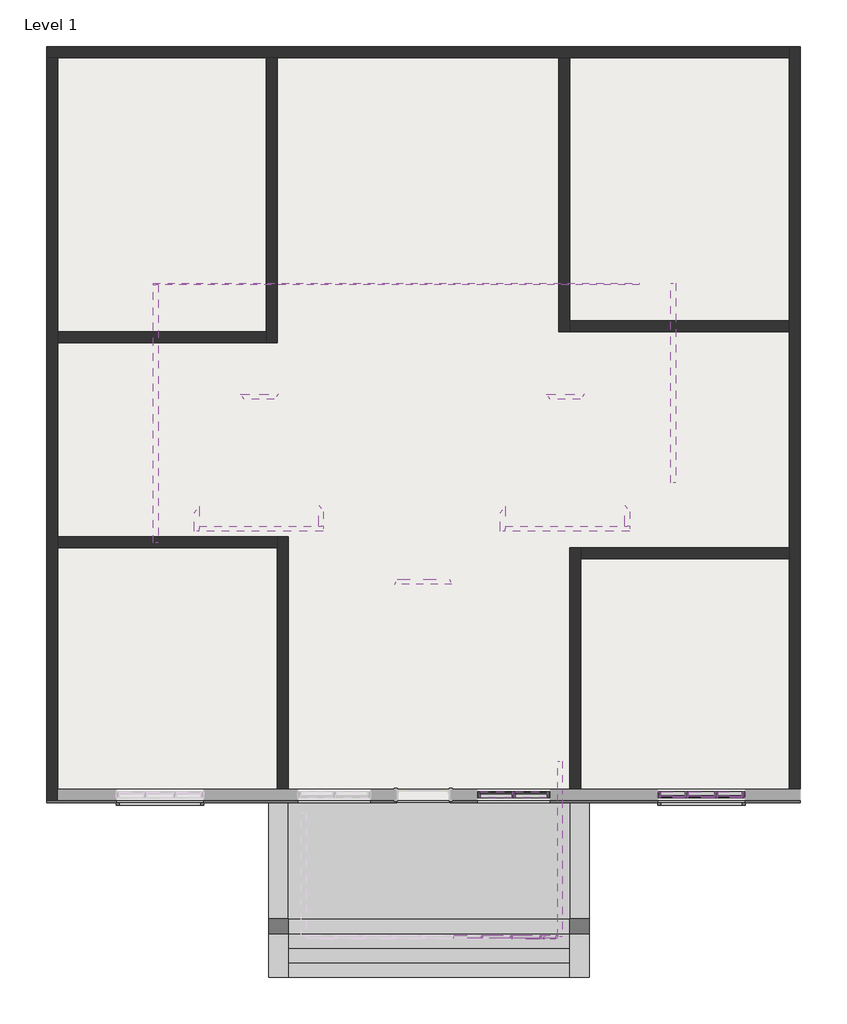
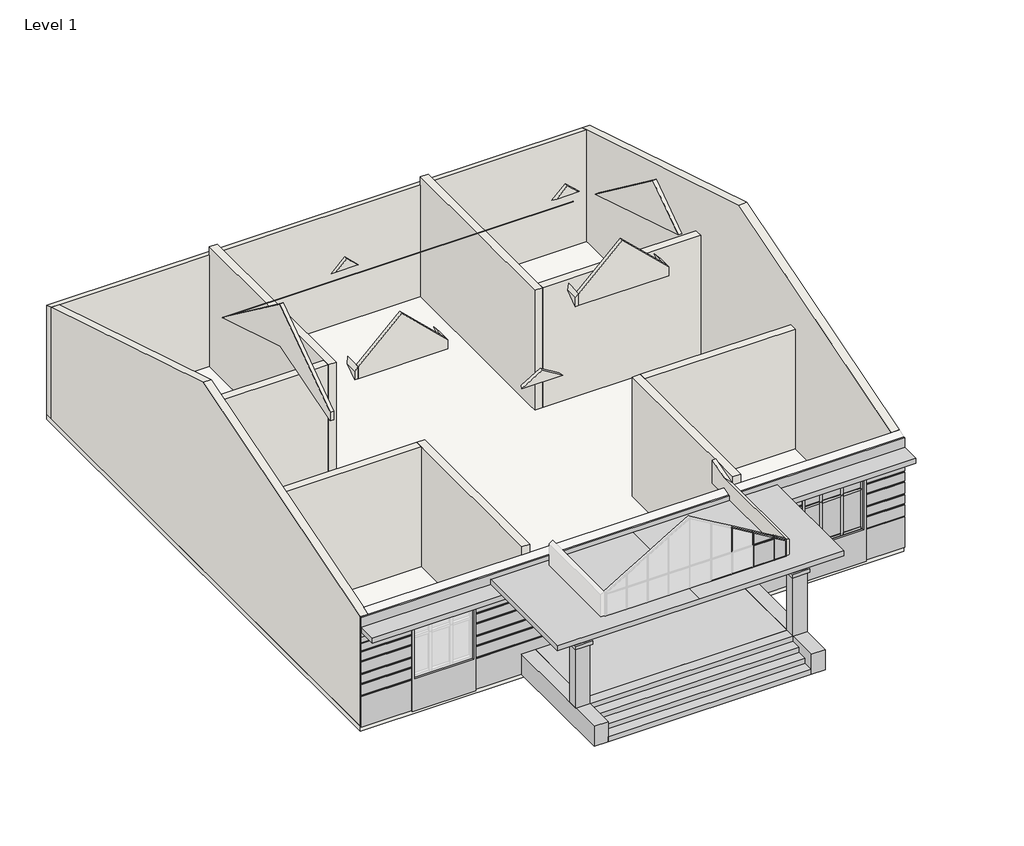
# One storey, part 2 of 2: 38 members, 24 walls, 11 plates, 1 proxy, 1 slab.
"""IFC4 building model written with IfcOpenShell, lengths in millimetres."""

from ifc_helpers import new_model, si_unit, frame, origin, origin_with_axes, place, context, project, spatial, polyline, outline, extrude, faceted_brep, transform, mapped, element, save
from components import generic_models_1_generic_models_1_130779d0, member_b22cb31b, member_1ff0c156, member_6458fcce, member_a67f877f, member_f89b2291, member_594eddbe, member_fdc2508a, member_99ded25b, member_354dc74f, member_6356c2c7, member_864d0aaa, member_0b7646a3, member_2b49869a, member_aaa03826, member_0a1a1ade, member_a980948f, member_6e77e263, member_47bfaf8a, member_75074519, member_c33c434a, member_38e9bff8, member_062c1ce8, system_panel_glazed_d796fc41, system_panel_glazed_2d0a2ff2, system_panel_glazed_c086748d, system_panel_glazed_4278ab3a, system_panel_glazed_31f7001e, system_panel_glazed_2554e476, system_panel_glazed_f02c31ce, system_panel_glazed_28184e5f

model = new_model("IFC4")

# Units and contexts
model_context = context("Model", 3, world=origin())
ifc_project = project(units=[si_unit("LENGTHUNIT", "METRE", prefix="MILLI")], contexts=[model_context])

# Site, building, storey
site = spatial("IfcSite", under=ifc_project)
building = spatial("IfcBuilding", under=site)
storey = spatial("IfcBuildingStorey", under=building, Name="Level 1", Elevation=0.0)

# Proxy
placement = place(None, origin())
generic_models_1_generic_models_1_shape = generic_models_1_generic_models_1_130779d0(model_context)
element("IfcBuildingElementProxy", 1, Name="Generic Models 1 : Generic Models 1", ObjectType="Generic Models 1 : Generic Models 1", at=placement, inside=storey, context=model_context, shape_type="MappedRepresentation", body=[
    mapped(generic_models_1_generic_models_1_shape, transform((0.0, 0.0, 0.0), x_axis=(1.0, 0.0, 0.0), y_axis=(0.0, 1.0, 0.0), z_axis=(0.0, 0.0, 1.0))),
])

# Members
member_shape = member_b22cb31b(model_context)
element("IfcMember", 2, ObjectType="Rectangular Mullion : 1.5\" x 2.5\" rectangular", at=placement, inside=storey, context=model_context, shape_type="MappedRepresentation", body=[
    mapped(member_shape, transform((1849.2182444, -4522.7940778, 3200.4), x_axis=(0.0, 0.0, -1.0), y_axis=(0.0, 1.0, 0.0), z_axis=(1.0, 0.0, 0.0))),
])
member_2_shape = member_1ff0c156(model_context)
element("IfcMember", 3, ObjectType="Rectangular Mullion : 1.5\" x 2.5\" rectangular", at=placement, inside=storey, context=model_context, shape_type="MappedRepresentation", body=[
    mapped(member_2_shape, transform((1551.6847658, -4522.7940778, 3886.2), x_axis=(0.0, 0.0, 1.0), y_axis=(0.0, 1.0, 0.0), z_axis=(-1.0, 0.0, 0.0))),
])
member_3_shape = member_6458fcce(model_context)
element("IfcMember", 4, ObjectType="Rectangular Mullion : 1.5\" x 2.5\" rectangular", at=placement, inside=storey, context=model_context, shape_type="MappedRepresentation", body=[
    mapped(member_3_shape, transform((1532.6347658, -4522.7940778, 3200.4), x_axis=(-1.0, 0.0, 0.0), y_axis=(0.0, 1.0, 0.0), z_axis=(0.0, 0.0, -1.0))),
])
member_4_shape = member_a67f877f(model_context)
element("IfcMember", 5, ObjectType="Rectangular Mullion : 1.5\" x 2.5\" rectangular", at=placement, inside=storey, context=model_context, shape_type="MappedRepresentation", body=[
    mapped(member_4_shape, transform((294.3847658, -4522.7940778, 3200.4), x_axis=(0.0, 0.0, -1.0), y_axis=(0.0, 1.0, 0.0), z_axis=(1.0, 0.0, 0.0))),
])
element("IfcMember", 6, ObjectType="Rectangular Mullion : 1.5\" x 2.5\" rectangular", at=placement, inside=storey, context=model_context, shape_type="MappedRepresentation", body=[
    mapped(member_4_shape, transform((903.9847658, -4522.7940778, 3200.4), x_axis=(0.0, 0.0, -1.0), y_axis=(0.0, 1.0, 0.0), z_axis=(1.0, 0.0, 0.0))),
])
element("IfcMember", 7, ObjectType="Rectangular Mullion : 1.5\" x 2.5\" rectangular", at=placement, inside=storey, context=model_context, shape_type="MappedRepresentation", body=[
    mapped(member_4_shape, transform((1513.5847658, -4522.7940778, 3200.4), x_axis=(0.0, 0.0, -1.0), y_axis=(0.0, 1.0, 0.0), z_axis=(1.0, 0.0, 0.0))),
])
member_5_shape = member_f89b2291(model_context)
element("IfcMember", 8, ObjectType="Rectangular Mullion : 1.5\" x 2.5\" rectangular", at=placement, inside=storey, context=model_context, shape_type="MappedRepresentation", body=[
    mapped(member_5_shape, transform((1617.4006914, -4522.7940778, 3886.2), x_axis=(0.5109163571310299, 0.0, 0.8596304299034312), y_axis=(0.0, 1.0, 0.0), z_axis=(-0.8596304299034312, 0.0, 0.5109163571310299))),
])
member_6_shape = member_594eddbe(model_context)
element("IfcMember", 9, ObjectType="Rectangular Mullion : 1.5\" x 2.5\" rectangular", at=placement, inside=storey, context=model_context, shape_type="MappedRepresentation", body=[
    mapped(member_6_shape, transform((313.4347658, -4522.7940778, 4661.2045803), x_axis=(0.5109163571310306, 0.0, 0.8596304299034309), y_axis=(0.0, 1.0, 0.0), z_axis=(-0.8596304299034307, 0.0, 0.5109163571310305))),
])
element("IfcMember", 10, ObjectType="Rectangular Mullion : 1.5\" x 2.5\" rectangular", at=placement, inside=storey, context=model_context, shape_type="MappedRepresentation", body=[
    mapped(member_6_shape, transform((923.0347658, -4522.7940778, 4298.8923581), x_axis=(0.5109163571310307, 0.0, 0.8596304299034307), y_axis=(0.0, 1.0, 0.0), z_axis=(-0.8596304299034307, 0.0, 0.5109163571310307))),
])
member_7_shape = member_fdc2508a(model_context)
element("IfcMember", 11, ObjectType="Rectangular Mullion : 1.5\" x 2.5\" rectangular", at=placement, inside=storey, context=model_context, shape_type="MappedRepresentation", body=[
    mapped(member_7_shape, transform((1532.6347658, -4522.7940778, 3936.5801359), x_axis=(0.5109163571310298, 0.0, 0.8596304299034313), y_axis=(0.0, 1.0, 0.0), z_axis=(-0.8596304299034312, 0.0, 0.5109163571310297))),
])
member_8_shape = member_99ded25b(model_context)
element("IfcMember", 12, ObjectType="Rectangular Mullion : 1.5\" x 2.5\" rectangular", at=placement, inside=storey, context=model_context, shape_type="MappedRepresentation", body=[
    mapped(member_8_shape, transform((313.4347658, -4522.7940778, 3886.2), x_axis=(-1.0, 0.0, 0.0), y_axis=(0.0, 1.0, 0.0), z_axis=(0.0, 0.0, -1.0))),
])
member_9_shape = member_354dc74f(model_context)
element("IfcMember", 13, ObjectType="Rectangular Mullion : 1.5\" x 2.5\" rectangular", at=placement, inside=storey, context=model_context, shape_type="MappedRepresentation", body=[
    mapped(member_9_shape, transform((923.0347658, -4522.7940778, 3886.2), x_axis=(-1.0, 0.0, 0.0), y_axis=(0.0, 1.0, 0.0), z_axis=(0.0, 0.0, -1.0))),
])
member_10_shape = member_6356c2c7(model_context)
element("IfcMember", 14, ObjectType="Rectangular Mullion : 1.5\" x 2.5\" rectangular", at=placement, inside=storey, context=model_context, shape_type="MappedRepresentation", body=[
    mapped(member_10_shape, transform((1532.6347658, -4522.7940778, 3886.2), x_axis=(-1.0, 0.0, 0.0), y_axis=(0.0, 1.0, 0.0), z_axis=(0.0, 0.0, -1.0))),
])
member_11_shape = member_864d0aaa(model_context)
element("IfcMember", 15, ObjectType="Rectangular Mullion : 1.5\" x 2.5\" rectangular", at=placement, inside=storey, context=model_context, shape_type="MappedRepresentation", body=[
    mapped(member_11_shape, transform((1887.3182444, -4522.7940778, 3725.7760689), x_axis=(1.0, 0.0, 0.0), y_axis=(0.0, 1.0, 0.0), z_axis=(0.0, 0.0, 1.0))),
])
member_12_shape = member_0b7646a3(model_context)
element("IfcMember", 16, ObjectType="Rectangular Mullion : 2.5\" x 5\" rectangular", at=placement, inside=storey, context=model_context, shape_type="MappedRepresentation", body=[
    mapped(member_12_shape, transform((4034.5347658, -1562.8594336, 2743.2), x_axis=(0.0, 0.0, 1.0), y_axis=(0.0, 1.0, 0.0), z_axis=(-1.0, 0.0, 0.0))),
])
element("IfcMember", 17, ObjectType="Rectangular Mullion : 2.5\" x 5\" rectangular", at=placement, inside=storey, context=model_context, shape_type="MappedRepresentation", body=[
    mapped(member_12_shape, transform((5221.9847658, -1562.8594336, 2743.2), x_axis=(0.0, 0.0, 1.0), y_axis=(0.0, 1.0, 0.0), z_axis=(-1.0, 0.0, 0.0))),
])
element("IfcMember", 18, ObjectType="Rectangular Mullion : 2.5\" x 5\" rectangular", at=placement, inside=storey, context=model_context, shape_type="MappedRepresentation", body=[
    mapped(member_12_shape, transform((5736.3347658, -1562.8594336, 914.4), x_axis=(0.0, 0.0, -1.0), y_axis=(0.0, 1.0, 0.0), z_axis=(1.0, 0.0, 0.0))),
])
element("IfcMember", 19, ObjectType="Rectangular Mullion : 2.5\" x 5\" rectangular", at=placement, inside=storey, context=model_context, shape_type="MappedRepresentation", body=[
    mapped(member_12_shape, transform((4548.8847658, -1562.8594336, 914.4), x_axis=(0.0, 0.0, -1.0), y_axis=(0.0, 1.0, 0.0), z_axis=(1.0, 0.0, 0.0))),
])
member_13_shape = member_2b49869a(model_context)
element("IfcMember", 20, ObjectType="Rectangular Mullion : 2.5\" x 5\" rectangular", at=placement, inside=storey, context=model_context, shape_type="MappedRepresentation", body=[
    mapped(member_13_shape, transform((4580.6347658, -1562.8594336, 914.4), x_axis=(-1.0, 0.0, 0.0), y_axis=(0.0, 1.0, 0.0), z_axis=(0.0, 0.0, -1.0))),
])
element("IfcMember", 21, ObjectType="Rectangular Mullion : 2.5\" x 5\" rectangular", at=placement, inside=storey, context=model_context, shape_type="MappedRepresentation", body=[
    mapped(member_13_shape, transform((5190.2347658, -1562.8594336, 914.4), x_axis=(-1.0, 0.0, 0.0), y_axis=(0.0, 1.0, 0.0), z_axis=(0.0, 0.0, -1.0))),
])
member_14_shape = member_aaa03826(model_context)
element("IfcMember", 22, ObjectType="Rectangular Mullion : 2.5\" x 5\" rectangular", at=placement, inside=storey, context=model_context, shape_type="MappedRepresentation", body=[
    mapped(member_14_shape, transform((5221.9847658, -1562.8594336, 2133.6), x_axis=(0.0, 0.0, 1.0), y_axis=(0.0, 1.0, 0.0), z_axis=(-1.0, 0.0, 0.0))),
])
element("IfcMember", 23, ObjectType="Rectangular Mullion : 2.5\" x 5\" rectangular", at=placement, inside=storey, context=model_context, shape_type="MappedRepresentation", body=[
    mapped(member_14_shape, transform((4034.5347658, -1562.8594336, 2133.6), x_axis=(0.0, 0.0, 1.0), y_axis=(0.0, 1.0, 0.0), z_axis=(-1.0, 0.0, 0.0))),
])
member_15_shape = member_0a1a1ade(model_context)
element("IfcMember", 24, ObjectType="Rectangular Mullion : 2.5\" x 5\" rectangular", at=placement, inside=storey, context=model_context, shape_type="MappedRepresentation", body=[
    mapped(member_15_shape, transform((4612.3847658, -1562.8594336, 2133.6), x_axis=(0.0, 0.0, 1.0), y_axis=(0.0, 1.0, 0.0), z_axis=(-1.0, 0.0, 0.0))),
])
member_16_shape = member_a980948f(model_context)
element("IfcMember", 25, ObjectType="Rectangular Mullion : 2.5\" x 5\" rectangular", at=placement, inside=storey, context=model_context, shape_type="MappedRepresentation", body=[
    mapped(member_16_shape, transform((5158.4847658, -1562.8594336, 914.4), x_axis=(0.0, 0.0, -1.0), y_axis=(0.0, 1.0, 0.0), z_axis=(1.0, 0.0, 0.0))),
])
element("IfcMember", 26, ObjectType="Rectangular Mullion : 2.5\" x 5\" rectangular", at=placement, inside=storey, context=model_context, shape_type="MappedRepresentation", body=[
    mapped(member_16_shape, transform((4612.3847658, -1562.8594336, 2743.2), x_axis=(0.0, 0.0, 1.0), y_axis=(0.0, 1.0, 0.0), z_axis=(-1.0, 0.0, 0.0))),
])
member_17_shape = member_6e77e263(model_context)
element("IfcMember", 27, ObjectType="Rectangular Mullion : 2.5\" x 5\" rectangular", at=placement, inside=storey, context=model_context, shape_type="MappedRepresentation", body=[
    mapped(member_17_shape, transform((4580.6347658, -1562.8594336, 2133.6), x_axis=(-1.0, 0.0, 0.0), y_axis=(0.0, 1.0, 0.0), z_axis=(0.0, 0.0, -1.0))),
])
element("IfcMember", 28, ObjectType="Rectangular Mullion : 2.5\" x 5\" rectangular", at=placement, inside=storey, context=model_context, shape_type="MappedRepresentation", body=[
    mapped(member_17_shape, transform((5190.2347658, -1562.8594336, 2133.6), x_axis=(-1.0, 0.0, 0.0), y_axis=(0.0, 1.0, 0.0), z_axis=(0.0, 0.0, -1.0))),
])
member_18_shape = member_47bfaf8a(model_context)
element("IfcMember", 29, ObjectType="Rectangular Mullion : 2.5\" x 5\" rectangular", at=placement, inside=storey, context=model_context, shape_type="MappedRepresentation", body=[
    mapped(member_18_shape, transform((5799.8347658, -1562.8594336, 2743.2), x_axis=(1.0, 0.0, 0.0), y_axis=(0.0, 1.0, 0.0), z_axis=(0.0, 0.0, 1.0))),
])
member_19_shape = member_75074519(model_context)
element("IfcMember", 30, ObjectType="Rectangular Mullion : 2.5\" x 5\" rectangular", at=placement, inside=storey, context=model_context, shape_type="MappedRepresentation", body=[
    mapped(member_19_shape, transform((3971.0347658, -1562.8594336, 914.4), x_axis=(-1.0, 0.0, 0.0), y_axis=(0.0, 1.0, 0.0), z_axis=(0.0, 0.0, -1.0))),
])
element("IfcMember", 31, ObjectType="Rectangular Mullion : 2.5\" x 5\" rectangular", at=placement, inside=storey, context=model_context, shape_type="MappedRepresentation", body=[
    mapped(member_18_shape, transform((3971.0347658, -1562.8594336, 2133.6), x_axis=(-1.0, 0.0, 0.0), y_axis=(0.0, 1.0, 0.0), z_axis=(0.0, 0.0, -1.0))),
])
element("IfcMember", 32, ObjectType="Rectangular Mullion : 2.5\" x 5\" rectangular", at=placement, inside=storey, context=model_context, shape_type="MappedRepresentation", body=[
    mapped(member_19_shape, transform((5799.8347658, -1562.8594336, 2133.6), x_axis=(1.0, 0.0, 0.0), y_axis=(0.0, 1.0, 0.0), z_axis=(0.0, 0.0, 1.0))),
])
member_20_shape = member_c33c434a(model_context)
element("IfcMember", 33, ObjectType="Rectangular Mullion : 2.5\" x 5\" rectangular", at=placement, inside=storey, context=model_context, shape_type="MappedRepresentation", body=[
    mapped(member_20_shape, transform((1672.3347658, -1562.8594336, 2743.2), x_axis=(0.0, 0.0, 1.0), y_axis=(0.0, -1.0, 0.0), z_axis=(1.0, 0.0, 0.0))),
])
element("IfcMember", 34, ObjectType="Rectangular Mullion : 2.5\" x 5\" rectangular", at=placement, inside=storey, context=model_context, shape_type="MappedRepresentation", body=[
    mapped(member_20_shape, transform((942.0847658, -1562.8594336, 2743.2), x_axis=(0.0, 0.0, 1.0), y_axis=(0.0, -1.0, 0.0), z_axis=(1.0, 0.0, 0.0))),
])
element("IfcMember", 35, ObjectType="Rectangular Mullion : 2.5\" x 5\" rectangular", at=placement, inside=storey, context=model_context, shape_type="MappedRepresentation", body=[
    mapped(member_20_shape, transform((275.3347658, -1562.8594336, 1066.8), x_axis=(0.0, 0.0, -1.0), y_axis=(0.0, -1.0, 0.0), z_axis=(-1.0, 0.0, 0.0))),
])
element("IfcMember", 36, ObjectType="Rectangular Mullion : 2.5\" x 5\" rectangular", at=placement, inside=storey, context=model_context, shape_type="MappedRepresentation", body=[
    mapped(member_20_shape, transform((1005.5847658, -1562.8594336, 1066.8), x_axis=(0.0, 0.0, -1.0), y_axis=(0.0, -1.0, 0.0), z_axis=(-1.0, 0.0, 0.0))),
])
member_21_shape = member_38e9bff8(model_context)
element("IfcMember", 37, ObjectType="Rectangular Mullion : 2.5\" x 5\" rectangular", at=placement, inside=storey, context=model_context, shape_type="MappedRepresentation", body=[
    mapped(member_21_shape, transform((973.8347658, -1562.8594336, 1066.8), x_axis=(1.0, 0.0, 0.0), y_axis=(0.0, -1.0, 0.0), z_axis=(0.0, 0.0, -1.0))),
])
member_22_shape = member_062c1ce8(model_context)
element("IfcMember", 38, ObjectType="Rectangular Mullion : 2.5\" x 5\" rectangular", at=placement, inside=storey, context=model_context, shape_type="MappedRepresentation", body=[
    mapped(member_22_shape, transform((211.8347658, -1562.8594336, 2743.2), x_axis=(-1.0, 0.0, 0.0), y_axis=(0.0, -1.0, 0.0), z_axis=(0.0, 0.0, 1.0))),
])
element("IfcMember", 39, ObjectType="Rectangular Mullion : 2.5\" x 5\" rectangular", at=placement, inside=storey, context=model_context, shape_type="MappedRepresentation", body=[
    mapped(member_22_shape, transform((1735.8347658, -1562.8594336, 1066.8), x_axis=(1.0, 0.0, 0.0), y_axis=(0.0, -1.0, 0.0), z_axis=(0.0, 0.0, -1.0))),
])

# Plates
system_panel_glazed_shape = system_panel_glazed_d796fc41(model_context)
element("IfcPlate", 40, ObjectType="System Panel : Glazed", at=placement, inside=storey, context=model_context, shape_type="MappedRepresentation", body=[
    mapped(system_panel_glazed_shape, transform((5479.1597658, -1562.8594336, 977.9), x_axis=(-1.0, 0.0, 0.0), y_axis=(0.0, -1.0, 0.0), z_axis=(0.0, 0.0, 1.0))),
])
element("IfcPlate", 41, ObjectType="System Panel : Glazed", at=placement, inside=storey, context=model_context, shape_type="MappedRepresentation", body=[
    mapped(system_panel_glazed_shape, transform((4291.7097658, -1562.8594336, 977.9), x_axis=(-1.0, 0.0, 0.0), y_axis=(0.0, -1.0, 0.0), z_axis=(0.0, 0.0, 1.0))),
])
system_panel_glazed_2_shape = system_panel_glazed_2d0a2ff2(model_context)
element("IfcPlate", 42, ObjectType="System Panel : Glazed", at=placement, inside=storey, context=model_context, shape_type="MappedRepresentation", body=[
    mapped(system_panel_glazed_2_shape, transform((4885.4347658, -1562.8594336, 977.9), x_axis=(-1.0, 0.0, 0.0), y_axis=(0.0, -1.0, 0.0), z_axis=(0.0, 0.0, 1.0))),
])
system_panel_glazed_3_shape = system_panel_glazed_c086748d(model_context)
element("IfcPlate", 43, ObjectType="System Panel : Glazed", at=placement, inside=storey, context=model_context, shape_type="MappedRepresentation", body=[
    mapped(system_panel_glazed_3_shape, transform((5479.1597658, -1562.8594336, 2165.35), x_axis=(-1.0, 0.0, 0.0), y_axis=(0.0, -1.0, 0.0), z_axis=(0.0, 0.0, 1.0))),
])
element("IfcPlate", 44, ObjectType="System Panel : Glazed", at=placement, inside=storey, context=model_context, shape_type="MappedRepresentation", body=[
    mapped(system_panel_glazed_3_shape, transform((4291.7097658, -1562.8594336, 2165.35), x_axis=(-1.0, 0.0, 0.0), y_axis=(0.0, -1.0, 0.0), z_axis=(0.0, 0.0, 1.0))),
])
system_panel_glazed_4_shape = system_panel_glazed_4278ab3a(model_context)
element("IfcPlate", 45, ObjectType="System Panel : Glazed", at=placement, inside=storey, context=model_context, shape_type="MappedRepresentation", body=[
    mapped(system_panel_glazed_4_shape, transform((4885.4347658, -1562.8594336, 2165.35), x_axis=(-1.0, 0.0, 0.0), y_axis=(0.0, -1.0, 0.0), z_axis=(0.0, 0.0, 1.0))),
])
system_panel_glazed_5_shape = system_panel_glazed_31f7001e(model_context)
element("IfcPlate", 46, ObjectType="System Panel : Glazed", at=placement, inside=storey, context=model_context, shape_type="MappedRepresentation", body=[
    mapped(system_panel_glazed_5_shape, transform((608.7097658, -1562.8594336, 1130.3), x_axis=(1.0, 0.0, 0.0), y_axis=(0.0, 1.0, 0.0), z_axis=(0.0, 0.0, 1.0))),
])
element("IfcPlate", 47, ObjectType="System Panel : Glazed", at=placement, inside=storey, context=model_context, shape_type="MappedRepresentation", body=[
    mapped(system_panel_glazed_5_shape, transform((1338.9597658, -1562.8594336, 1130.3), x_axis=(1.0, 0.0, 0.0), y_axis=(0.0, 1.0, 0.0), z_axis=(0.0, 0.0, 1.0))),
])
system_panel_glazed_6_shape = system_panel_glazed_2554e476(model_context)
element("IfcPlate", 48, ObjectType="System Panel : Glazed", at=placement, inside=storey, context=model_context, shape_type="MappedRepresentation", body=[
    mapped(system_panel_glazed_6_shape, transform((1700.4515051, -4522.7940778, 3238.5), x_axis=(-1.0, 0.0, 0.0), y_axis=(0.0, -1.0, 0.0), z_axis=(0.0, 0.0, 1.0))),
])
system_panel_glazed_7_shape = system_panel_glazed_f02c31ce(model_context)
element("IfcPlate", 49, ObjectType="System Panel : Glazed", at=placement, inside=storey, context=model_context, shape_type="MappedRepresentation", body=[
    mapped(system_panel_glazed_7_shape, transform((1227.8347658, -4522.7940778, 3238.5), x_axis=(-1.0, 0.0, 0.0), y_axis=(0.0, -1.0, 0.0), z_axis=(0.0, 0.0, 1.0))),
])
system_panel_glazed_8_shape = system_panel_glazed_28184e5f(model_context)
element("IfcPlate", 50, ObjectType="System Panel : Glazed", at=placement, inside=storey, context=model_context, shape_type="MappedRepresentation", body=[
    mapped(system_panel_glazed_8_shape, transform((1226.4307149, -4522.7940778, 3905.25), x_axis=(-1.0, 0.0, 0.0), y_axis=(0.0, -1.0, 0.0), z_axis=(0.0, 0.0, 1.0))),
])

# Slab
element("IfcSlab", 51, ObjectType="6\" floor", at=placement, inside=storey, context=model_context, shape_type="SweptSolid", body=[
    extrude(outline(polyline([(-8754.3652342, 14020.0405664), (6942.8347658, 14020.0405664), (6942.8347658, -1677.1594336), (-8754.3652342, -1677.1594336), (-8754.3652342, 14020.0405664)])), frame((0.0, 0.0, -152.4), z_axis=(0.0, 0.0, 1.0), x_axis=(1.0, 0.0, 0.0)), (0.0, 0.0, 1.0), 152.4),
])

# Walls
element("IfcWall", 52, ObjectType="4\" wall", at=placement, inside=storey, context=model_context, shape_type="Brep", body=[
    faceted_brep([(-310.6134198, 2818.6405664, 5032.1039977), (-905.7652342, 2818.6405664, 5385.8290246), (-1500.9170486, 2818.6405664, 5032.1039977), (-1448.654004, 2920.2405664, 5063.1662349), (-905.7652342, 2920.2405664, 5385.8290246), (-362.8764644, 2920.2405664, 5063.1662349)], [[[0, 1, 2]], [[3, 4, 5]], [[0, 2, 3, 5]], [[2, 1, 4, 3]], [[1, 0, 5, 4]]]),
])
element("IfcWall", 53, ObjectType="4\" wall", at=placement, inside=storey, context=model_context, shape_type="Brep", body=[
    faceted_brep([(1887.3182444, -4522.7940778, 3200.4), (1887.3182444, -4522.7940778, 3725.7760689), (1887.3182444, -1454.1655602, 3725.7760689), (1887.3182444, -865.1940778, 3905.8427215), (1887.3182444, -865.1940778, 3200.4), (1887.3182444, -1448.5594336, 3200.4), (1887.3182444, -1448.5594336, 3408.7631864), (1887.3182444, -1677.1594336, 3338.8731526), (1887.3182444, -1677.1594336, 3200.4), (1988.9182444, -4522.7940778, 3665.3906985), (1988.9182444, -4522.7940778, 3200.4), (1988.9182444, -1677.1594336, 3200.4), (1988.9182444, -1677.1594336, 3338.8731526), (1988.9182444, -1448.5594336, 3408.7631864), (1988.9182444, -1448.5594336, 3200.4), (1988.9182444, -865.1940778, 3200.4), (1988.9182444, -865.1940778, 3905.8427215), (1988.9182444, -1651.677207, 3665.3906985)], [[[0, 1, 2, 3, 4, 5, 6, 7, 8]], [[9, 10, 11, 12, 13, 14, 15, 16, 17]], [[10, 0, 8, 11]], [[4, 15, 14, 5]], [[1, 0, 10, 9]], [[4, 3, 16, 15]], [[13, 6, 5, 14]], [[7, 12, 11, 8]], [[16, 3, 2, 17]], [[1, 9, 17, 2]], [[6, 13, 12, 7]]]),
])
element("IfcWall", 54, ObjectType="4\" wall", at=placement, inside=storey, context=model_context, shape_type="Brep", body=[
    faceted_brep([(3590.0347658, 9058.6011476, 5189.588834), (-6428.4074718, 9058.6011476, 5189.588834), (-6530.0074718, 9058.6011476, 5189.588834), (-6530.0074718, 9058.6011476, 5174.4642545), (-6428.4074718, 9058.6011476, 5174.4642545), (3590.0347658, 9058.6011476, 5174.4642545), (3590.0347658, 9092.704913, 5164.0376871), (-6530.0074718, 9092.704913, 5164.0376871)], [[[0, 1, 2, 3, 4, 5]], [[0, 5, 6]], [[3, 2, 7]], [[2, 1, 0, 6, 7]], [[5, 4, 3, 7, 6]]]),
])
element("IfcWall", 55, ObjectType="4\" wall", at=placement, inside=storey, context=model_context, shape_type="SweptSolid", body=[
    extrude(outline(polyline([(3682.2405664, 5296.1330142), (3682.2405664, 5557.4858701), (6207.4951043, 7325.6881334), (9058.6011476, 5189.588834), (9058.6011476, 5174.4642545), (6171.4405664, 6057.1578265), (3682.2405664, 5296.1330142)])), frame((-6530.0074718, 0.0, 0.0), z_axis=(1.0, 0.0, 0.0), x_axis=(0.0, 1.0, 0.0)), (0.0, 0.0, 1.0), 101.6),
])
element("IfcWall", 56, ObjectType="4\" wall", at=placement, inside=storey, context=model_context, shape_type="SweptSolid", body=[
    extrude(outline(polyline([(4935.4952336, 6435.0242353), (6207.4951043, 7325.6881334), (9092.704913, 5164.0376871), (4935.4952336, 6435.0242353)])), frame((4250.4347658, 0.0, 0.0), z_axis=(1.0, 0.0, 0.0), x_axis=(0.0, 1.0, 0.0)), (0.0, 0.0, 1.0), 101.6),
])
element("IfcWall", 57, ObjectType="4\" wall", at=placement, inside=storey, context=model_context, shape_type="Brep", body=[
    faceted_brep([(-4010.4112278, 6671.251642, 7359.0904892), (-4324.604279, 6671.251642, 7658.5050511), (-4638.7973302, 6671.251642, 7359.0904892), (-4718.6750083, 6772.851642, 7282.9699642), (-4324.604279, 6772.851642, 7658.5050511), (-3930.5335497, 6772.851642, 7282.9699642)], [[[0, 1, 2]], [[3, 4, 5]], [[1, 4, 3, 2]], [[4, 1, 0, 5]], [[0, 2, 3, 5]]]),
])
element("IfcWall", 58, ObjectType="4\" wall", at=placement, inside=storey, context=model_context, shape_type="Brep", body=[
    faceted_brep([(-5578.199649, 4445.2946862, 6463.8742114), (-5578.199649, 4029.651642, 6463.8742114), (-5578.199649, 3928.051642, 6463.8742114), (-5578.199649, 3928.051642, 6101.6967329), (-5578.199649, 4029.651642, 6172.8378187), (-5679.799649, 3928.051642, 6101.6967329), (-5679.799649, 3928.051642, 6367.053103), (-5679.799649, 4307.0198131, 6367.053103)], [[[0, 1, 2, 3, 4]], [[5, 6, 7]], [[2, 6, 5, 3]], [[6, 2, 1, 0, 7]], [[0, 4, 3, 5, 7]]]),
])
element("IfcWall", 59, ObjectType="4\" wall", at=placement, inside=storey, context=model_context, shape_type="Brep", body=[
    faceted_brep([(-2987.399649, 4029.651642, 6172.8378187), (-3088.999649, 4029.651642, 6172.8378187), (-5578.199649, 4029.651642, 6172.8378187), (-5578.199649, 4029.651642, 6463.8742114), (-4324.604279, 4029.651642, 7658.5050511), (-3088.999649, 4029.651642, 6481.018733), (-2987.399649, 4029.651642, 6384.1976246), (-2987.399649, 3928.051642, 6101.6967329), (-2987.399649, 3928.051642, 6384.1976246), (-4324.604279, 3928.051642, 7658.5050511), (-5578.199649, 3928.051642, 6463.8742114), (-5578.199649, 3928.051642, 6101.6967329)], [[[0, 1, 2, 3, 4, 5, 6]], [[7, 8, 9, 10, 11]], [[0, 6, 8, 7]], [[3, 2, 11, 10]], [[6, 5, 4, 9, 8]], [[4, 3, 10, 9]], [[2, 1, 0, 7, 11]]]),
])
element("IfcWall", 60, ObjectType="4\" wall", at=placement, inside=storey, context=model_context, shape_type="Brep", body=[
    faceted_brep([(-3088.999649, 4029.651642, 6172.8378187), (-3088.999649, 4029.651642, 6481.018733), (-3088.999649, 4469.7796005, 6481.018733), (-2987.399649, 4331.5047274, 6384.1976246), (-2987.399649, 4029.651642, 6384.1976246), (-2987.399649, 4029.651642, 6172.8378187)], [[[0, 1, 2]], [[3, 4, 5]], [[4, 1, 0, 5]], [[1, 4, 3, 2]], [[0, 2, 3, 5]]]),
])
element("IfcWall", 61, ObjectType="4\" wall", at=placement, inside=storey, context=model_context, shape_type="Brep", body=[
    faceted_brep([(2364.758858, 6671.251642, 7359.0904892), (2050.5658068, 6671.251642, 7658.5050511), (1736.3727556, 6671.251642, 7359.0904892), (1656.4950775, 6772.851642, 7282.9699642), (2050.5658068, 6772.851642, 7658.5050511), (2444.6365361, 6772.851642, 7282.9699642)], [[[0, 1, 2]], [[3, 4, 5]], [[1, 4, 3, 2]], [[4, 1, 0, 5]], [[0, 2, 3, 5]]]),
])
element("IfcWall", 62, ObjectType="4\" wall", at=placement, inside=storey, context=model_context, shape_type="Brep", body=[
    faceted_brep([(796.9704368, 4445.2946862, 6463.8742114), (796.9704368, 4029.651642, 6463.8742114), (796.9704368, 3928.051642, 6463.8742114), (796.9704368, 3928.051642, 6101.6967329), (796.9704368, 4029.651642, 6172.8378187), (695.3704368, 3928.051642, 6101.6967329), (695.3704368, 3928.051642, 6367.053103), (695.3704368, 4307.0198131, 6367.053103)], [[[0, 1, 2, 3, 4]], [[5, 6, 7]], [[2, 6, 5, 3]], [[6, 2, 1, 0, 7]], [[0, 4, 3, 5, 7]]]),
])
element("IfcWall", 63, ObjectType="4\" wall", at=placement, inside=storey, context=model_context, shape_type="Brep", body=[
    faceted_brep([(3387.7704368, 4029.651642, 6172.8378187), (3286.1704368, 4029.651642, 6172.8378187), (796.9704368, 4029.651642, 6172.8378187), (796.9704368, 4029.651642, 6463.8742114), (2050.5658068, 4029.651642, 7658.5050511), (3286.1704368, 4029.651642, 6481.018733), (3387.7704368, 4029.651642, 6384.1976246), (3387.7704368, 3928.051642, 6101.6967329), (3387.7704368, 3928.051642, 6384.1976246), (2050.5658068, 3928.051642, 7658.5050511), (796.9704368, 3928.051642, 6463.8742114), (796.9704368, 3928.051642, 6101.6967329)], [[[0, 1, 2, 3, 4, 5, 6]], [[7, 8, 9, 10, 11]], [[0, 6, 8, 7]], [[3, 2, 11, 10]], [[6, 5, 4, 9, 8]], [[4, 3, 10, 9]], [[2, 1, 0, 7, 11]]]),
])
element("IfcWall", 64, ObjectType="4\" wall", at=placement, inside=storey, context=model_context, shape_type="Brep", body=[
    faceted_brep([(3286.1704368, 4029.651642, 6172.8378187), (3286.1704368, 4029.651642, 6481.018733), (3286.1704368, 4469.7796005, 6481.018733), (3387.7704368, 4331.5047274, 6384.1976246), (3387.7704368, 4029.651642, 6384.1976246), (3387.7704368, 4029.651642, 6172.8378187)], [[[0, 1, 2]], [[3, 4, 5]], [[4, 1, 0, 5]], [[1, 4, 3, 2]], [[0, 2, 3, 5]]]),
])
element("IfcWall", 65, ObjectType="9\"", at=placement, inside=storey, context=model_context, shape_type="Brep", body=[
    faceted_brep([(-8754.3652342, 13791.4405664, 0.0), (-8525.7652342, 13791.4405664, 0.0), (-4182.3652342, 13791.4405664, 0.0), (-3953.7652342, 13791.4405664, 0.0), (1913.6347658, 13791.4405664, 0.0), (2142.2347658, 13791.4405664, 0.0), (6714.2347658, 13791.4405664, 0.0), (6714.2347658, 13791.4405664, 3408.7631864), (-8525.7652342, 13791.4405664, 3408.7631864), (-8754.3652342, 13791.4405664, 3408.7631864), (-8754.3652342, 14020.0405664, 0.0), (-8754.3652342, 14020.0405664, 3338.8731526), (6714.2347658, 14020.0405664, 3338.8731526), (6714.2347658, 14020.0405664, 0.0)], [[[0, 1, 2, 3, 4, 5, 6, 7, 8, 9]], [[10, 11, 12, 13]], [[6, 5, 4, 3, 2, 1, 0, 10, 13]], [[0, 9, 11, 10]], [[7, 6, 13, 12]], [[9, 8, 7, 12, 11]]]),
])
element("IfcWall", 66, ObjectType="9\"", at=placement, inside=storey, context=model_context, shape_type="Brep", body=[
    faceted_brep([(-8525.7652342, -1677.1594336, 0.0), (-8525.7652342, -1448.5594336, 0.0), (-8525.7652342, 3580.6405664, 0.0), (-8525.7652342, 3809.2405664, 0.0), (-8525.7652342, 7847.8405664, 0.0), (-8525.7652342, 8076.4405664, 0.0), (-8525.7652342, 13791.4405664, 0.0), (-8525.7652342, 13791.4405664, 3408.7631864), (-8525.7652342, 6171.4405664, 5738.4309791), (-8525.7652342, -1448.5594336, 3408.7631864), (-8525.7652342, -1677.1594336, 3338.8731526), (-8754.3652342, -1677.1594336, 0.0), (-8754.3652342, -1677.1594336, 3338.8731526), (-8754.3652342, 6171.4405664, 5738.4309791), (-8754.3652342, 13791.4405664, 3408.7631864), (-8754.3652342, 13791.4405664, 0.0)], [[[0, 1, 2, 3, 4, 5, 6, 7, 8, 9, 10]], [[11, 12, 13, 14, 15]], [[6, 5, 4, 3, 2, 1, 0, 11, 15]], [[0, 10, 12, 11]], [[7, 6, 15, 14]], [[10, 9, 8, 13, 12]], [[8, 7, 14, 13]]]),
])
element("IfcWall", 67, ObjectType="9\"", at=placement, inside=storey, context=model_context, shape_type="Brep", body=[
    faceted_brep([(6714.2347658, 14020.0405664, 0.0), (6714.2347658, 13791.4405664, 0.0), (6714.2347658, 8305.0405664, 0.0), (6714.2347658, 8076.4405664, 0.0), (6714.2347658, 3580.6405664, 0.0), (6714.2347658, 3352.0405664, 0.0), (6714.2347658, -1448.5594336, 0.0), (6714.2347658, -1448.5594336, 3408.7631864), (6714.2347658, 6171.4405664, 5738.4309791), (6714.2347658, 13791.4405664, 3408.7631864), (6714.2347658, 14020.0405664, 3338.8731526), (6942.8347658, 14020.0405664, 0.0), (6942.8347658, 14020.0405664, 3338.8731526), (6942.8347658, 6171.4405664, 5738.4309791), (6942.8347658, -1448.5594336, 3408.7631864), (6942.8347658, -1448.5594336, 0.0)], [[[0, 1, 2, 3, 4, 5, 6, 7, 8, 9, 10]], [[11, 12, 13, 14, 15]], [[6, 5, 4, 3, 2, 1, 0, 11, 15]], [[0, 10, 12, 11]], [[7, 6, 15, 14]], [[10, 9, 8, 13, 12]], [[8, 7, 14, 13]]]),
])
element("IfcWall", 68, ObjectType="9\"", at=placement, inside=storey, context=model_context, shape_type="SweptSolid", body=[
    extrude(outline(polyline([(6714.2347658, 3352.0405664), (2370.8347658, 3352.0405664), (2370.8347658, 3580.6405664), (6714.2347658, 3580.6405664), (6714.2347658, 3352.0405664)])), origin_with_axes(), (0.0, 0.0, 1.0), 3657.6),
])
element("IfcWall", 69, ObjectType="9\"", at=placement, inside=storey, context=model_context, shape_type="SweptSolid", body=[
    extrude(outline(polyline([(-8525.7652342, 3809.2405664), (-3953.7652342, 3809.2405664), (-3953.7652342, 3580.6405664), (-8525.7652342, 3580.6405664), (-8525.7652342, 3809.2405664)])), origin_with_axes(), (0.0, 0.0, 1.0), 3657.6),
])
element("IfcWall", 70, ObjectType="9\"", at=placement, inside=storey, context=model_context, shape_type="Brep", body=[
    faceted_brep([(-4182.3652342, 13791.4405664, 0.0), (-4182.3652342, 8076.4405664, 0.0), (-4182.3652342, 7847.8405664, 0.0), (-4182.3652342, 7847.8405664, 3657.6), (-4182.3652342, 8076.4405664, 3657.6), (-4182.3652342, 13791.4405664, 3657.6), (-3953.7652342, 13791.4405664, 0.0), (-3953.7652342, 13791.4405664, 3657.6), (-3953.7652342, 7847.8405664, 3657.6), (-3953.7652342, 7847.8405664, 0.0)], [[[0, 1, 2, 3, 4, 5]], [[6, 7, 8, 9]], [[2, 1, 0, 6, 9]], [[5, 4, 3, 8, 7]], [[0, 5, 7, 6]], [[3, 2, 9, 8]]]),
])
element("IfcWall", 71, ObjectType="9\"", at=placement, inside=storey, context=model_context, shape_type="Brep", body=[
    faceted_brep([(1913.6347658, 13791.4405664, 0.0), (1913.6347658, 8076.4405664, 0.0), (1913.6347658, 8076.4405664, 3657.6), (1913.6347658, 13791.4405664, 3657.6), (2142.2347658, 13791.4405664, 0.0), (2142.2347658, 13791.4405664, 3657.6), (2142.2347658, 8305.0405664, 3657.6), (2142.2347658, 8076.4405664, 3657.6), (2142.2347658, 8076.4405664, 0.0), (2142.2347658, 8305.0405664, 0.0)], [[[0, 1, 2, 3]], [[4, 5, 6, 7, 8, 9]], [[1, 0, 4, 9, 8]], [[3, 2, 7, 6, 5]], [[0, 3, 5, 4]], [[2, 1, 8, 7]]]),
])
element("IfcWall", 72, ObjectType="9\"", at=placement, inside=storey, context=model_context, shape_type="SweptSolid", body=[
    extrude(outline(polyline([(2142.2347658, 8305.0405664), (6714.2347658, 8305.0405664), (6714.2347658, 8076.4405664), (2142.2347658, 8076.4405664), (2142.2347658, 8305.0405664)])), origin_with_axes(), (0.0, 0.0, 1.0), 3657.6),
])
element("IfcWall", 73, ObjectType="9\"", at=placement, inside=storey, context=model_context, shape_type="SweptSolid", body=[
    extrude(outline(polyline([(-4182.3652342, 7847.8405664), (-8525.7652342, 7847.8405664), (-8525.7652342, 8076.4405664), (-4182.3652342, 8076.4405664), (-4182.3652342, 7847.8405664)])), origin_with_axes(), (0.0, 0.0, 1.0), 3657.6),
])
element("IfcWall", 74, ObjectType="9\"", at=placement, inside=storey, context=model_context, shape_type="Brep", body=[
    faceted_brep([(-3725.1652342, -1448.5594336, 0.0), (-3725.1652342, 3809.2405664, 0.0), (-3725.1652342, 3809.2405664, 3657.6), (-3725.1652342, -1448.5594336, 3657.6), (-3953.7652342, -1448.5594336, 0.0), (-3953.7652342, -1448.5594336, 3657.6), (-3953.7652342, 3580.6405664, 3657.6), (-3953.7652342, 3809.2405664, 3657.6), (-3953.7652342, 3809.2405664, 0.0), (-3953.7652342, 3580.6405664, 0.0)], [[[0, 1, 2, 3]], [[4, 5, 6, 7, 8, 9]], [[1, 0, 4, 9, 8]], [[3, 2, 7, 6, 5]], [[2, 1, 8, 7]], [[0, 3, 5, 4]]]),
])
element("IfcWall", 75, ObjectType="9\"", at=placement, inside=storey, context=model_context, shape_type="Brep", body=[
    faceted_brep([(2370.8347658, -1448.5594336, 0.0), (2370.8347658, 3352.0405664, 0.0), (2370.8347658, 3580.6405664, 0.0), (2370.8347658, 3580.6405664, 3657.6), (2370.8347658, 3352.0405664, 3657.6), (2370.8347658, -1448.5594336, 3657.6), (2142.2347658, -1448.5594336, 0.0), (2142.2347658, -1448.5594336, 3657.6), (2142.2347658, 3580.6405664, 3657.6), (2142.2347658, 3580.6405664, 0.0)], [[[0, 1, 2, 3, 4, 5]], [[6, 7, 8, 9]], [[2, 1, 0, 6, 9]], [[5, 4, 3, 8, 7]], [[3, 2, 9, 8]], [[0, 5, 7, 6]]]),
])

save(model, "model.ifc")

# Revit data of these elements
# Type "Rectangular Mullion : 1.5\" x 2.5\" rectangular"
#   built-in parameter 1007304 = 0.208333 (stored number, unit not read)
#   built-in parameter 1007301 = 0.0625 (stored number, unit not read)
#   built-in parameter 1007300 = 0.0625 (stored number, unit not read)
# Type "Rectangular Mullion : 2.5\" x 5\" rectangular"
#   built-in parameter 1007304 = 0.416667 (stored number, unit not read)
#   built-in parameter 1007301 = 0.104167 (stored number, unit not read)
#   built-in parameter 1007300 = 0.104167 (stored number, unit not read)
# Type "System Panel : Glazed"
#   Construction Type Id = "GSP4R"
#   Analytic Construction = "1/8 in Pilkington single glazing"
#   Visual Light Transmittance = 0.9
#   Solar Heat Gain Coefficient = 0.86
#   Heat Transfer Coefficient (U) = 1.18115 BTU/(h·ft²·°F)
#   Define Thermal Properties by = 1
# Type "6\" floor"
#   Assembly Code = "B1010"
#   Function = 0
#   Layers, outside or top first: 0' - 6" no material (function 1)
# Type "4\" wall"
#   Assembly Code = "B2010"
#   Layers, outside or top first: 0' - 4" "Gypsum Wall Board" (function 1)
# Type "9\""
#   Assembly Code = "B2010"
#   Layers, outside or top first: 0' - 9" "Gypsum Wall Board" (function 1)
# Element 1 (IfcBuildingElementProxy, "Generic Models 1 : Generic Models 1")
#   Phase Created = New Construction
#   Materials on its faces: "Gypsum Wall Board", "rock b"
# Elements 2, 3, 4, 5, 6, 7, 8, 9, 10, 11, 12, 13, 14, 15 (IfcMember, "Rectangular Mullion : 1.5\" x 2.5\" rectangular")
#   Phase Created = New Construction
# Elements 16, 17, 18, 19, 20, 21, 22, 23, 24, 25, 26, 27, 28, 29, 30, 31, 32, 33, 34, 35, 36, 37, 38, 39 (IfcMember, "Rectangular Mullion : 2.5\" x 5\" rectangular")
#   Phase Created = New Construction
# Elements 40, 41, 42, 43, 44, 45, 46, 47, 48, 49, 50 (IfcPlate, "System Panel : Glazed")
#   Phase Created = New Construction
#   Materials on its faces: "Glass"
# Element 51 (IfcSlab, "6\" floor")
#   built-in parameter 1001955 = 3.14159 (stored number, unit not read)
#   Height Offset From Level = 0' - 0"
#   Phase Created = New Construction
#   Materials on its faces: "Default Floor"
# Element 52 (IfcWall, "4\" wall")
#   built-in parameter 1001111 = 2' - 0"
#   Top Offset = -3' - 0"
#   Base Offset = 2' - 0"
#   wall height = 7' - 0"
#   Phase Created = New Construction
#   Base Constraint = Level 1
#   Top Constraint = Level 2
#   Materials on its faces: "Gypsum Wall Board"
# Element 53 (IfcWall, "4\" wall")
#   built-in parameter 1001111 = 10' - 6"
#   Top Offset = -3' - 0"
#   Base Offset = 10' - 6"
#   wall height = 7' - 0"
#   Phase Created = New Construction
#   Base Constraint = Level 1
#   Top Constraint = Level 2
#   Materials on its faces: "Gypsum Wall Board"
# Elements 54, 55, 56, 57, 58, 59, 60, 61, 62, 63, 64 (IfcWall, "4\" wall")
#   built-in parameter 1001111 = 2' - 0"
#   Top Offset = -3' - 0"
#   Base Offset = 2' - 0"
#   Unconnected Height = 7' - 0"
#   wall height = 7' - 0"
#   Phase Created = New Construction
#   Base Constraint = Level 1
#   Materials on its faces: "Gypsum Wall Board"
# Elements 65, 66, 67, 68, 69, 70, 71, 72, 73, 74, 75 (IfcWall, "9\"")
#   Top Offset = 0' - 0"
#   Base Offset = 0' - 0"
#   wall height = 12' - 0"
#   Phase Created = New Construction
#   Base Constraint = Level 1
#   Top Constraint = Level 2
#   Materials on its faces: "Gypsum Wall Board"
# Materials
#   "Gypsum Wall Board": class "Generic", colour RGB 127 127 127, transparency 0, Description = "Gypsum Wall Board", Cost = 0
#   "rock b": class "Generic", colour RGB 120 120 120, transparency 0, Cost = 0
#   "Glass": class "Glass", colour RGB 0 128 192, transparency 0.75, Description = "Soda Lime Glass", Cost = 0
#   "Default Floor": colour RGB 128 128 128, transparency 0, Cost = 0
